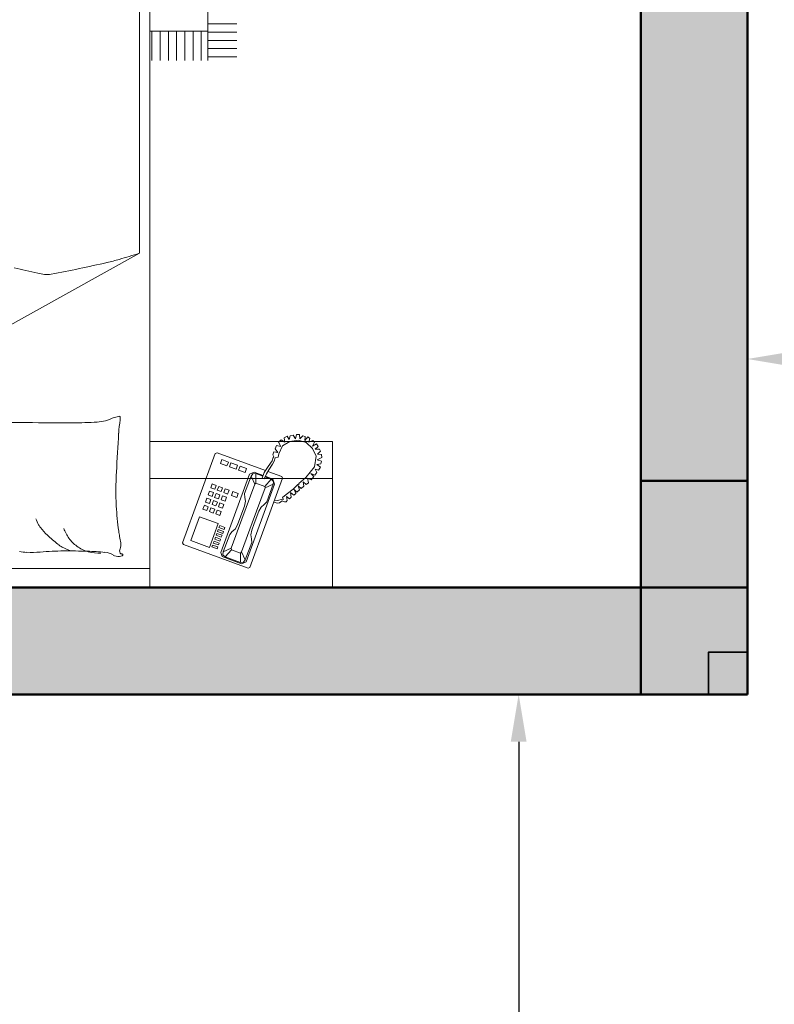
# Model space of a CAD drawing. Units: inches. Extents: x -7 to 1228, y -146 to 1091.
# Tile 37 of 88: x 1066 to 1129, y 34 to 117. Entities that reach past the tile are written whole.
import ezdxf

# ---------------------------------------------------------------- set-up
doc = ezdxf.new("R2010")
doc.units = ezdxf.units.IN
for name, color, linetype, lineweight in [('A-ANNO-DIMS', 2, 'Continuous', 18), ('A-COLS', 6, 'Continuous', 35), ('A-FURN', 8, 'Continuous', 18), ('A-WALL', 7, 'Continuous', 50), ('A-WALL-PATT', 251, 'Continuous', 13)]:
    doc.layers.add(name, color=color, linetype=linetype, lineweight=lineweight)
doc.styles.add('DIM_FONT', font='SIMPLEX.shx', dxfattribs={"width": 0.8})
doc.styles.get("Standard").update_dxf_attribs({"font": 'arial.ttf'})
doc.dimstyles.new('ISO-25', dxfattribs={"dimtxt": 7, "dimasz": 4, "dimexe": 1.25, "dimexo": 0.625, "dimtad": 1, "dimdec": 1, "dimlunit": 3, "dimtxsty": 'Standard', "dimcen": 2.5, "dimadec": 0, "dimazin": 0, "dimtfac": 1, "dimtdec": 1, "dimtmove": 1, "dimatfit": 3, "dimfxl": 1, "dimarcsym": 0})

# ---------------------------------------------------------------- blocks, each defined once
blk = doc.blocks.new('A$C4F634EDD')
for p, q in [((0.5, 2.6295), (2.3, 2.6295)), ((2.3, 2.6295), (2.3, 0.5295)), ((2.3, 2.6295), (2.8, 2.6295)), ((2.3, 2.2295), (2.3, 2.6295)), ((2.8, 2.6295), (2.8, 2.2295)), ((0.5, 2.5771), (2.3, 2.5771)), ((2.392, 2.5115), (2.5692, 2.5765)), ((2.4985, 2.5445), (2.5516, 2.564)), ((2.5516, 2.564), (2.5637, 2.5584)), ((2.5692, 2.5765), (2.574, 2.5743)), ((2.574, 2.5743), (2.6638, 2.3298)), ((2.4946, 2.5331), (2.4985, 2.5445)), ((2.5062, 2.5454), (2.5004, 2.5392)), ((2.5004, 2.5392), (2.5013, 2.5315)), ((2.5062, 2.5454), (2.5487, 2.561)), ((2.5235, 2.5256), (2.5062, 2.5454)), ((2.5483, 2.5347), (2.5487, 2.561)), ((2.5487, 2.561), (2.5571, 2.56)), ((2.5615, 2.5536), (2.5514, 2.5318)), ((2.5571, 2.56), (2.5615, 2.5536)), ((2.5615, 2.5536), (2.5791, 2.5058)), ((2.5637, 2.5584), (2.6418, 2.3458)), ((2.3898, 2.5066), (2.392, 2.5115)), ((2.412, 2.5007), (2.4634, 2.5196)), ((2.4634, 2.5196), (2.4875, 2.454)), ((2.4842, 2.5232), (2.47, 2.518)), ((2.47, 2.518), (2.472, 2.5127)), ((2.472, 2.5127), (2.4862, 2.5179)), ((2.4881, 2.5126), (2.4739, 2.5074)), ((2.4862, 2.5179), (2.4842, 2.5232)), ((2.4901, 2.5073), (2.4881, 2.5126)), ((2.5734, 2.3187), (2.4946, 2.5331)), ((2.5013, 2.5315), (2.5188, 2.4836)), ((2.5013, 2.5315), (2.5231, 2.5214)), ((2.5231, 2.5214), (2.5235, 2.5256)), ((2.5523, 2.4417), (2.5231, 2.5214)), ((2.5483, 2.5347), (2.5235, 2.5256)), ((2.5514, 2.5318), (2.5483, 2.5347)), ((2.5807, 2.4521), (2.5514, 2.5318)), ((2.4795, 2.2621), (2.3898, 2.5066)), ((2.4361, 2.4352), (2.412, 2.5007)), ((2.4739, 2.5074), (2.4759, 2.502)), ((2.4759, 2.502), (2.4901, 2.5073)), ((2.492, 2.5019), (2.4778, 2.4967)), ((2.4778, 2.4967), (2.4798, 2.4914)), ((2.4798, 2.4914), (2.494, 2.4966)), ((2.4959, 2.4913), (2.4817, 2.4861)), ((2.4817, 2.4861), (2.4837, 2.4808)), ((2.4837, 2.4808), (2.4979, 2.486)), ((2.494, 2.4966), (2.492, 2.5019)), ((2.4979, 2.486), (2.4959, 2.4913)), ((2.5188, 2.4836), (2.5256, 2.4761)), ((2.5788, 2.4956), (2.5767, 2.4848)), ((2.5767, 2.4848), (2.5795, 2.4717)), ((2.5791, 2.5058), (2.5788, 2.4956)), ((2.4998, 2.4807), (2.4856, 2.4755)), ((2.4856, 2.4755), (2.4876, 2.4702)), ((2.4876, 2.4702), (2.5018, 2.4754)), ((2.5037, 2.47), (2.4895, 2.4648)), ((2.4895, 2.4648), (2.4915, 2.4595)), ((2.4915, 2.4595), (2.5057, 2.4647)), ((2.5018, 2.4754), (2.4998, 2.4807)), ((2.5057, 2.4647), (2.5037, 2.47)), ((2.5256, 2.4761), (2.5342, 2.4692)), ((2.5342, 2.4692), (2.5405, 2.4574)), ((2.5405, 2.4574), (2.547, 2.4397)), ((2.5795, 2.4717), (2.586, 2.454)), ((2.4875, 2.454), (2.4361, 2.4352)), ((2.4811, 2.4276), (2.4917, 2.4315)), ((2.485, 2.4169), (2.4811, 2.4276)), ((2.4917, 2.4315), (2.4956, 2.4208)), ((2.5594, 2.4061), (2.547, 2.4397)), ((2.5523, 2.4417), (2.5875, 2.346)), ((2.5807, 2.4521), (2.6158, 2.3564)), ((2.5984, 2.4204), (2.586, 2.454)), ((2.4457, 2.4146), (2.4563, 2.4185)), ((2.4496, 2.4039), (2.4457, 2.4146)), ((2.4602, 2.4078), (2.4496, 2.4039)), ((2.4563, 2.4185), (2.4602, 2.4078)), ((2.4634, 2.4211), (2.474, 2.425)), ((2.4673, 2.4104), (2.4634, 2.4211)), ((2.4779, 2.4143), (2.4673, 2.4104)), ((2.4706, 2.4016), (2.4812, 2.4055)), ((2.4745, 2.3909), (2.4706, 2.4016)), ((2.474, 2.425), (2.4779, 2.4143)), ((2.4812, 2.4055), (2.4851, 2.3949)), ((2.4956, 2.4208), (2.485, 2.4169)), ((2.4883, 2.4081), (2.4989, 2.412)), ((2.4922, 2.3975), (2.4883, 2.4081)), ((2.5028, 2.4014), (2.4922, 2.3975)), ((2.4989, 2.412), (2.5028, 2.4014)), ((2.5622, 2.393), (2.5594, 2.4061)), ((2.6047, 2.4086), (2.5984, 2.4204)), ((2.6133, 2.4017), (2.6047, 2.4086)), ((2.6201, 2.3941), (2.6133, 2.4017)), ((2.4528, 2.3951), (2.4635, 2.399)), ((2.4567, 2.3844), (2.4528, 2.3951)), ((2.4674, 2.3883), (2.4567, 2.3844)), ((2.46, 2.3756), (2.4706, 2.3795)), ((2.4639, 2.365), (2.46, 2.3756)), ((2.4635, 2.399), (2.4674, 2.3883)), ((2.4706, 2.3795), (2.4745, 2.3689)), ((2.4851, 2.3949), (2.4745, 2.3909)), ((2.4777, 2.3821), (2.4883, 2.386)), ((2.4816, 2.3715), (2.4777, 2.3821)), ((2.4922, 2.3754), (2.4816, 2.3715)), ((2.4883, 2.386), (2.4922, 2.3754)), ((2.4954, 2.3886), (2.5061, 2.3925)), ((2.4993, 2.378), (2.4954, 2.3886)), ((2.51, 2.3819), (2.4993, 2.378)), ((2.5061, 2.3925), (2.51, 2.3819)), ((2.5238, 2.3769), (2.538, 2.3821)), ((2.5277, 2.3663), (2.5238, 2.3769)), ((2.538, 2.3821), (2.5419, 2.3715)), ((2.5598, 2.372), (2.5601, 2.3822)), ((2.5601, 2.3822), (2.5622, 2.393)), ((2.6376, 2.3463), (2.6201, 2.3941)), ((2.6499, 2.3979), (2.6397, 2.3953)), ((2.6417, 2.39), (2.6488, 2.391)), ((2.6488, 2.391), (2.6538, 2.3895)), ((2.6551, 2.397), (2.6499, 2.3979)), ((2.6538, 2.3895), (2.6596, 2.388)), ((2.6627, 2.392), (2.6551, 2.397)), ((2.6596, 2.388), (2.6626, 2.3867)), ((2.6626, 2.3867), (2.6662, 2.388)), ((2.6692, 2.394), (2.6627, 2.392)), ((2.6662, 2.388), (2.6632, 2.3828)), ((2.6632, 2.3828), (2.6736, 2.3744)), ((2.6736, 2.3944), (2.6692, 2.394)), ((2.6765, 2.391), (2.6736, 2.3944)), ((2.6736, 2.3744), (2.6922, 2.3593)), ((2.6742, 2.3795), (2.6765, 2.391)), ((2.6824, 2.3858), (2.6742, 2.3795)), ((2.6873, 2.3815), (2.6824, 2.3858)), ((2.6853, 2.369), (2.6873, 2.3815)), ((2.6946, 2.376), (2.6853, 2.369)), ((2.6995, 2.3713), (2.6946, 2.376)), ((2.4745, 2.3689), (2.4639, 2.365)), ((2.4672, 2.3561), (2.4778, 2.36)), ((2.4711, 2.3455), (2.4672, 2.3561)), ((2.4817, 2.3494), (2.4711, 2.3455)), ((2.4778, 2.36), (2.4817, 2.3494)), ((2.4849, 2.3626), (2.4955, 2.3665)), ((2.4888, 2.352), (2.4849, 2.3626)), ((2.4994, 2.3559), (2.4888, 2.352)), ((2.4955, 2.3665), (2.4994, 2.3559)), ((2.5026, 2.3691), (2.5132, 2.373)), ((2.5065, 2.3585), (2.5026, 2.3691)), ((2.5171, 2.3624), (2.5065, 2.3585)), ((2.5132, 2.373), (2.5171, 2.3624)), ((2.5419, 2.3715), (2.5277, 2.3663)), ((2.5774, 2.3242), (2.5598, 2.372)), ((2.6154, 2.3522), (2.5905, 2.3431)), ((2.6158, 2.3564), (2.6154, 2.3522)), ((2.6154, 2.3522), (2.6327, 2.3324)), ((2.6376, 2.3463), (2.6158, 2.3564)), ((2.6922, 2.3593), (2.7051, 2.3473)), ((2.695, 2.3603), (2.6995, 2.3713)), ((2.7031, 2.3682), (2.695, 2.3603)), ((2.7096, 2.3616), (2.7031, 2.3682)), ((2.7051, 2.3473), (2.7079, 2.3475)), ((2.7062, 2.351), (2.7096, 2.3616)), ((2.7147, 2.3578), (2.7062, 2.351)), ((2.7079, 2.3475), (2.7079, 2.3443)), ((2.7214, 2.3517), (2.7147, 2.3578)), ((2.7196, 2.34), (2.7214, 2.3517)), ((2.7286, 2.3466), (2.7196, 2.34)), ((2.7346, 2.3423), (2.7286, 2.3466)), ((2.8, 2.3301), (2.3, 2.3301)), ((2.5774, 2.3242), (2.5875, 2.346)), ((2.5818, 2.3178), (2.5774, 2.3242)), ((2.6104, 2.3222), (2.5855, 2.3131)), ((2.5875, 2.346), (2.5905, 2.3431)), ((2.5905, 2.3431), (2.5901, 2.3168)), ((2.5901, 2.3168), (2.6097, 2.324)), ((2.613, 2.3312), (2.6077, 2.3293)), ((2.6077, 2.3293), (2.6135, 2.3141)), ((2.6192, 2.3174), (2.613, 2.3312)), ((2.6153, 2.3261), (2.6327, 2.3324)), ((2.6369, 2.332), (2.6161, 2.3243)), ((2.6616, 2.3249), (2.6234, 2.3109)), ((2.6327, 2.3324), (2.6385, 2.3386)), ((2.6418, 2.3458), (2.6369, 2.332)), ((2.6385, 2.3386), (2.6376, 2.3463)), ((2.6638, 2.3298), (2.6616, 2.3249)), ((2.7079, 2.3443), (2.727, 2.3277)), ((2.727, 2.3277), (2.7512, 2.2983)), ((2.732, 2.3295), (2.7346, 2.3423)), ((2.7423, 2.3345), (2.732, 2.3295)), ((2.7406, 2.3172), (2.7495, 2.325)), ((2.7519, 2.3218), (2.7406, 2.3172)), ((2.7495, 2.325), (2.7423, 2.3345)), ((2.7575, 2.3144), (2.7519, 2.3218)), ((2.6172, 2.3086), (2.4844, 2.2599)), ((2.5114, 2.2959), (2.4936, 2.2894)), ((2.5153, 2.2853), (2.5114, 2.2959)), ((2.5362, 2.305), (2.5185, 2.2985)), ((2.5185, 2.2985), (2.5224, 2.2879)), ((2.5224, 2.2879), (2.5401, 2.2944)), ((2.5401, 2.2944), (2.5362, 2.305)), ((2.561, 2.3141), (2.5433, 2.3076)), ((2.5433, 2.3076), (2.5472, 2.297)), ((2.5472, 2.297), (2.5649, 2.3035)), ((2.5649, 2.3035), (2.561, 2.3141)), ((2.5855, 2.3131), (2.5734, 2.3187)), ((2.5901, 2.3168), (2.5818, 2.3178)), ((2.6135, 2.3141), (2.6244, 2.2977)), ((2.626, 2.3069), (2.6192, 2.3174)), ((2.6244, 2.2977), (2.6349, 2.2825)), ((2.6365, 2.2916), (2.626, 2.3069)), ((2.7512, 2.2983), (2.756, 2.2695)), ((2.7526, 2.3045), (2.7575, 2.3144)), ((2.7622, 2.308), (2.7526, 2.3045)), ((2.7574, 2.2924), (2.7673, 2.2997)), ((2.7673, 2.2997), (2.7622, 2.308)), ((2.4936, 2.2894), (2.4976, 2.2788)), ((2.4976, 2.2788), (2.5153, 2.2853)), ((2.6349, 2.2825), (2.638, 2.273)), ((2.6407, 2.2834), (2.6365, 2.2916)), ((2.6399, 2.2712), (2.6374, 2.2659)), ((2.6374, 2.2659), (2.6398, 2.257)), ((2.638, 2.273), (2.6399, 2.2712)), ((2.6438, 2.2739), (2.6407, 2.2834)), ((2.6519, 2.2716), (2.6438, 2.2739)), ((2.6535, 2.2628), (2.6519, 2.2716)), ((2.756, 2.2695), (2.7459, 2.2483)), ((2.7687, 2.2905), (2.7574, 2.2924)), ((2.7587, 2.279), (2.7699, 2.2828)), ((2.7708, 2.2725), (2.7587, 2.279)), ((2.7699, 2.2828), (2.7687, 2.2905)), ((2.7706, 2.2643), (2.7708, 2.2725)), ((2.4844, 2.2599), (2.4795, 2.2621)), ((2.6398, 2.257), (2.6509, 2.259)), ((2.6509, 2.259), (2.6431, 2.2492)), ((2.6431, 2.2492), (2.6473, 2.2398)), ((2.6473, 2.2398), (2.6592, 2.2429)), ((2.6592, 2.2429), (2.6521, 2.2314)), ((2.6636, 2.2409), (2.6535, 2.2628)), ((2.6836, 2.2287), (2.6636, 2.2409)), ((2.7459, 2.2483), (2.7284, 2.2317)), ((2.7509, 2.2314), (2.7459, 2.2418)), ((2.7459, 2.2418), (2.7568, 2.2352)), ((2.7529, 2.2505), (2.7645, 2.2498)), ((2.7607, 2.2424), (2.7529, 2.2505)), ((2.7568, 2.2352), (2.7607, 2.2424)), ((2.759, 2.2637), (2.7706, 2.2643)), ((2.7676, 2.2559), (2.759, 2.2637)), ((2.7645, 2.2498), (2.7676, 2.2559)), ((2.8, 2.2295), (2.3, 2.2295)), ((2.6521, 2.2314), (2.6598, 2.2248)), ((2.6598, 2.2248), (2.6697, 2.2309)), ((2.6697, 2.2309), (2.6684, 2.219)), ((2.6684, 2.219), (2.6761, 2.2145)), ((2.6761, 2.2145), (2.6821, 2.2237)), ((2.6821, 2.2237), (2.6843, 2.2135)), ((2.7063, 2.2256), (2.6836, 2.2287)), ((2.6843, 2.2135), (2.6927, 2.2117)), ((2.6927, 2.2117), (2.6986, 2.222)), ((2.6986, 2.222), (2.7019, 2.2098)), ((2.7284, 2.2317), (2.7063, 2.2256)), ((2.7102, 2.2104), (2.7113, 2.2218)), ((2.7113, 2.2218), (2.7192, 2.2137)), ((2.7192, 2.2137), (2.7255, 2.2152)), ((2.7255, 2.2152), (2.7242, 2.2265)), ((2.7242, 2.2265), (2.7324, 2.2165)), ((2.7324, 2.2165), (2.7386, 2.2208)), ((2.7386, 2.2208), (2.7354, 2.2306)), ((2.7354, 2.2306), (2.7462, 2.2264)), ((2.7462, 2.2264), (2.7509, 2.2314)), ((2.7019, 2.2098), (2.7102, 2.2104)), ((1.5035, 2.141), (2.2716, 1.7136)), ((2.2716, 0.5617), (2.2716, 1.7136)), ((2.3061, 1.1052), (2.3061, 1.1852)), ((2.3286, 1.1052), (2.3286, 1.1852)), ((2.3511, 1.1052), (2.3511, 1.1852)), ((2.3736, 1.1052), (2.3736, 1.1852)), ((2.3961, 1.1052), (2.3961, 1.1852)), ((2.4186, 1.1052), (2.4186, 1.1852)), ((2.4411, 1.1052), (2.4411, 1.1852)), ((2.4588, 1.1852), (2.4588, 0)), ((2.4588, 1.1753), (2.5388, 1.1753)), ((2.4588, 1.1528), (2.5388, 1.1528)), ((2.4588, 1.1303), (2.5388, 1.1303)), ((2.4588, 1.1078), (2.5388, 1.1078)), ((2.3, 1.1052), (2.4588, 1.1052)), ((2.4588, 1.0853), (2.5388, 1.0853))]:
    blk.add_line(p, q)
for centre, radius, start, end in [((2.1724, 2.5864), 0.0539, 275.2592, 300.6513), ((2.2146, 2.5152), 0.0289, 85.6975, 120.6513), ((2.2149, 2.519), 0.0251, 68.2117, 85.6975), ((2.2226, 2.533), 0.00428, 78.1069, 158.0096), ((2.224, 2.5395), 0.00232, 258.1069, 19.564), ((2.2229, 2.5391), 0.00342, 19.564, 68.2117), ((1.97, 2.3805), 0.1524, 92.5386, 100.1899), ((1.9761, 2.2433), 0.2897, 85.1982, 92.5386), ((2.0734, 3.4021), 0.8732, 265.1982, 269.4243), ((2.291, 2.2032), 0.3916, 128.3886, 133.8115), ((2.0954, 2.45), 0.0768, 117.2396, 128.3886), ((2.1674, 2.3102), 0.234, 110.8603, 117.2396), ((2.0797, 4.0232), 1.4943, 269.4243, 271.9079), ((2.1588, 2.4357), 0.0992, 126.0864, 143.8234), ((2.1588, 2.4357), 0.0992, 105.9352, 126.0864), ((2.1021, 3.3501), 0.8208, 271.9079, 275.2592), ((2.1588, 2.4357), 0.0992, 85.7841, 105.9352), ((2.2331, 2.5288), 0.0156, 158.0096, 201.421), ((2.1881, 2.5111), 0.0328, 351.8665, 21.421), ((2.1757, 2.3233), 0.2252, 133.8115, 140.9651), ((2.1588, 2.4357), 0.0992, 143.8234, 161.5603), ((2.4114, 2.448), 0.1983, 167.8905, 172.3191), ((1.977, 2.5413), 0.246, 347.8905, 351.8665), ((2.1719, 2.3625), 0.2002, 151.6832, 156.9972), ((2.0391, 2.4341), 0.0493, 140.9651, 151.6832), ((3.1198, 2.3525), 0.9131, 172.3191, 176.6313), ((2.8858, 2.3663), 0.6787, 176.6313, 181.6331), ((3.5721, 2.3859), 1.3652, 181.6331, 183.055), ((15.8249, 3.0398), 13.6356, 183.05496, 183.50486), ((2.5355, 2.2258), 0.3212, 183.5049, 189.9984), ((2.1093, -19.8405), 22.0183, 90.37908, 91.01965), ((2.0605, -3.5404), 5.7185, 89.7135, 90.9704), ((2.0833, 1.0141), 1.164, 86.426, 89.7135), ((2.1467, 2.0302), 0.1459, 77.131, 86.426), ((2.1691, 2.1283), 0.0453, 62.7159, 77.131), ((2.2251, 2.2367), 0.0767, 242.7159, 253.7788), ((2.2281, 2.247), 0.0875, 253.7788, 262.8796), ((2.2174, 2.1615), 0.00132, 262.8796, 343.3022), ((2.2001, 2.1667), 0.0193, 343.3022, 9.9984), ((1.4194, 4.2174), 2.5158, 281.6741, 283.1904), ((2.0378, 1.5789), 0.1942, 97.7304, 103.1904), ((2.0195, 1.7137), 0.0581, 79.2724, 97.7304), ((1.2737, -2.2227), 4.0646, 77.0745, 79.2724), ((2.0359, 1.0981), 0.6574, 74.0648, 77.0745), ((1.7125, -0.0344), 1.8351, 72.2636, 74.0648)]:
    blk.add_arc(centre, radius, start, end)
at = {"style": 'DIM_FONT', "width": 0.8, "flags": 9}
for tag, p in [('YSIZE', (0.5, 2.6295)), ('XSIZE', (0.5, 2.6295)), ('XSIZE', (2.2985, 2.6295)), ('YSIZE', (2.2985, 2.6295))]:
    blk.add_attdef(tag, p, '', height=0.0005, dxfattribs=at)
blk = doc.blocks.new('*D16')
at = {"layer": 'A-ANNO-DIMS', "color": 0, "lineweight": -2, "transparency": 16777216}
for p, q in [((1127, 88.082), (1127, 87.038)), ((1131, 88.288), (1183, 88.288)), ((1187, 88.082), (1187, 87.038))]:
    blk.add_line(p, q, dxfattribs=at)
at = {"layer": 'A-ANNO-DIMS', "color": 0, "transparency": 16777216}
for points in [[(1131, 88.955), (1131, 87.622), (1127, 88.288)], [(1183, 88.955), (1183, 87.622), (1187, 88.288)]]:
    blk.add_solid(points, dxfattribs=at)
at = {"layer": 'Defpoints', "color": 0, "transparency": 16777216}
for p in [(1127, 88.707), (1187, 88.707), (1187, 88.288)]:
    blk.add_point(p, dxfattribs=at)
at = {"layer": 'A-ANNO-DIMS', "color": 0, "transparency": 16777216, "insert": (1157, 92.473), "char_height": 7, "attachment_point": 5}
blk.add_mtext("5'", dxfattribs=at)
blk = doc.blocks.new('*D17')
at = {"layer": 'A-ANNO-DIMS', "color": 0, "lineweight": -2, "transparency": 16777216}
for p, q in [((1108.337, 60), (1108.962, 60)), ((1107.712, 56), (1107.712, 4)), ((1108.337, 0), (1108.962, 0))]:
    blk.add_line(p, q, dxfattribs=at)
at = {"layer": 'A-ANNO-DIMS', "color": 0, "transparency": 16777216}
for points in [[(1107.046, 56), (1108.379, 56), (1107.712, 60)], [(1107.046, 4), (1108.379, 4), (1107.712, 0)]]:
    blk.add_solid(points, dxfattribs=at)
at = {"layer": 'Defpoints', "color": 0, "transparency": 16777216}
for p in [(1107.712, 60), (1107.712, 0), (1107.712, 0)]:
    blk.add_point(p, dxfattribs=at)
at = {"layer": 'A-ANNO-DIMS', "color": 0, "transparency": 16777216, "insert": (1103.528, 30), "char_height": 7, "attachment_point": 5, "rotation": 90}
blk.add_mtext("5'", dxfattribs=at)

msp = doc.modelspace()

# ---------------------------------------------------------------- hatches: boundary and pattern name
at = {"layer": 'A-COLS'}
h = msp.add_hatch(color=256, dxfattribs=at)
h.dxf.hatch_style = 1
h.paths.add_polyline_path([(1127, 78), (1118, 78), (1118, 60), (1123.711, 60), (1123.711, 63.546), (1127, 63.546)])
h = msp.add_hatch(color=256, dxfattribs=at)
h.dxf.hatch_style = 1
h.paths.add_polyline_path([(1123.711, 63.546), (1123.711, 60), (1127, 60), (1127, 63.546)])
at = {"layer": 'A-WALL-PATT'}
h = msp.add_hatch(color=256, dxfattribs=at)
h.dxf.hatch_style = 1
h.paths.add_polyline_path([(69, 568), (60, 568), (60, 493), (63.289, 493), (69, 493)])
h.paths.add_polyline_path([(69, 662.405), (60, 662.405), (60, 586), (69, 586)], flags=17)
h.paths.add_polyline_path([(69, 723), (184, 723), (184, 734), (179, 734), (179, 728), (69, 728), (69, 741.623), (60, 741.623), (60, 698.405), (69, 698.405)], flags=17)
h.paths.add_polyline_path([(69, 782), (231, 782), (231, 728), (231, 723), (231, 586), (236, 586), (236, 787), (69, 787), (69, 800.126), (60, 800.126), (60, 765.623), (69, 765.623)])
h.paths.add_polyline_path([(184, 842), (189, 842), (189, 848), (173, 848), (173, 842), (179, 842), (179, 787), (184, 787)])
h.paths.add_polyline_path([(118.22, 69), (69, 69), (69, 60), (118.22, 60)])
h.paths.add_polyline_path([(227, 69), (154.22, 69), (154.22, 60), (227, 60)])
h.paths.add_polyline_path([(236, 60), (232.711, 60), (227, 60), (227, 36), (236, 36)])
h.paths.add_polyline_path([(389, 60), (380, 60), (380, 36), (389, 36)])
h.paths.add_polyline_path([(384, 181), (380, 181), (380, 115), (380, 78), (384, 78)])
h.paths.add_polyline_path([(380, 115), (334.547, 115), (334.547, 109), (380, 109)])
h.paths.add_polyline_path([(274.547, 115), (236, 115), (236, 201), (232.711, 201), (231, 201), (231, 78), (236, 78), (236, 109), (274.547, 109)])
h.paths.add_polyline_path([(69, 123), (60, 123), (60, 78), (69, 78)])
h.paths.add_polyline_path([(69, 201), (60, 201), (60, 159), (69, 159)])
h.paths.add_polyline_path([(143, 219), (69, 219), (69, 213), (143, 213)], flags=17)
h.paths.add_polyline_path([(189, 219), (184, 219), (184, 274), (231, 274), (231, 219), (236, 219), (236, 279), (184, 279), (184, 297), (179, 297), (179, 279), (69, 279), (69, 290.912), (60, 290.912), (60, 262.179), (69, 262.179), (69, 274), (179, 274), (179, 219), (173, 219), (173, 213), (189, 213)])
h.paths.add_polyline_path([(69, 238.179), (60, 238.179), (60, 219), (69, 219)], flags=17)
h.paths.add_polyline_path([(69, 333), (60, 333), (60, 314.912), (69, 314.912), (69, 316.965)])
h.paths.add_polyline_path([(190, 338), (184, 338), (69, 338), (69, 333), (179, 333), (179, 327), (184, 327), (184, 333.021), (190, 333.046)])
h.paths.add_polyline_path([(69, 386.806), (60, 386.806), (60, 351), (69, 351)])
h.paths.add_polyline_path([(69, 475), (60, 475), (60, 422.806), (69, 422.806)])
h.paths.add_polyline_path([(236, 475), (231, 475), (231, 351.238), (236, 351.238)])
h.paths.add_polyline_path([(384, 475), (380, 475), (380, 362), (384, 362)])
h.paths.add_polyline_path([(547, 307), (439, 307), (439, 356), (445, 356), (445, 362), (433, 362), (433, 307), (380, 307), (380, 244), (380, 241), (384, 241), (384, 301), (433, 301), (433, 277), (439, 277), (439, 301), (547, 301)])
h.paths.add_polyline_path([(547, 241), (439, 241), (439, 247), (433, 247), (433, 235), (547, 235)])
h.paths.add_polyline_path([(450, 69), (440.286, 69), (424.889, 69), (389, 69), (389, 60), (450, 60)])
h.paths.add_polyline_path([(547, 69), (486, 69), (486, 60), (547, 60)])
h.paths.add_polyline_path([(556, 148.268), (547, 148.268), (547, 78), (556, 78)])
h.paths.add_polyline_path([(556, 223), (547, 223), (547, 195), (547, 184.268), (556, 184.268)])
h.paths.add_polyline_path([(556, 311.192), (547, 311.192), (547, 273.075), (556, 273.075)])
h.paths.add_polyline_path([(556, 344), (552.711, 344), (547, 344), (547, 335.192), (556, 335.192)])
h.paths.add_polyline_path([(556, 249.075), (547, 249.075), (547, 241), (556, 241)])
h.paths.add_polyline_path([(547, 362), (475, 362), (475, 356), (547, 356)], flags=0)
h.paths.add_polyline_path([(556, 399.621), (547, 399.621), (547, 362), (556, 362)])
h.paths.add_polyline_path([(556, 475), (547, 475), (547, 435.621), (556, 435.621)])
h.paths.add_polyline_path([(547, 493), (389, 493), (389, 487), (547, 487)])
h.paths.add_polyline_path([(380, 493), (278, 493), (278, 487), (380, 487)])
h.paths.add_polyline_path([(227, 493), (69, 493), (69, 487), (227, 487)])
h.paths.add_polyline_path([(643, 122.445), (634, 122.445), (634, 78), (643, 78)])
h.paths.add_polyline_path([(702.5, 69), (692.786, 69), (677.389, 69), (643, 69), (643, 60), (702.5, 60)])
h.paths.add_polyline_path([(798, 69), (738.5, 69), (738.5, 60), (798, 60)])
h.paths.add_polyline_path([(807, 60), (803.711, 60), (798, 60), (798, 36), (807, 36)])
h.paths.add_polyline_path([(807, 109), (846.751, 109), (846.751, 115), (807, 115), (807, 159), (802, 159), (802, 78), (807, 78)])
h.paths.add_polyline_path([(807, 201), (802, 201), (802, 195), (807, 195)])
h.paths.add_polyline_path([(643, 201), (634, 201), (634, 158.445), (643, 158.445)])
h.paths.add_polyline_path([(756, 225), (751, 225), (751, 219), (643, 219), (643, 213), (756, 213)])
h.paths.add_polyline_path([(643, 240.848), (634, 240.848), (634, 219), (643, 219)])
h.paths.add_polyline_path([(643, 274), (643, 288.629), (634, 288.629), (634, 264.848), (643, 264.848)])
h.paths.add_polyline_path([(802, 279), (756, 279), (756, 297), (751, 297), (751, 279), (643, 279), (643, 274), (751, 274), (751, 255), (756, 255), (756, 274), (802, 274)])
h.paths.add_polyline_path([(807, 333), (803.711, 333), (802, 333), (802, 279), (802, 274), (802, 219), (807, 219)])
h.paths.add_polyline_path([(956, 182), (951, 182), (951, 115), (906.751, 115), (906.751, 109), (951, 109), (951, 78), (956, 78)])
h.paths.add_polyline_path([(960, 60), (951, 60), (951, 36), (960, 36)])
h.paths.add_polyline_path([(1021, 69), (1005.781, 69), (960, 69), (960, 60), (1021, 60)])
h.paths.add_polyline_path([(956, 224), (951, 224), (951, 218), (956, 218)])
h.paths.add_polyline_path([(956, 302), (1004, 302), (1004, 278), (1010, 278), (1010, 302), (1118, 302), (1118, 290.809), (1127, 290.809), (1127, 326.968), (1118, 326.968), (1118, 320.966), (1118, 307), (1010, 307), (1010, 356), (1016, 356), (1016, 362), (1004, 362), (1004, 307), (951, 307), (951, 244), (951, 242), (954.289, 242), (956, 242)])
h.paths.add_polyline_path([(643, 333), (634, 333), (634, 312.629), (643, 312.629), (643, 316.965)])
h.paths.add_polyline_path([(756, 338), (643, 338), (643, 333), (751, 333), (751, 327), (756, 327)])
h.paths.add_polyline_path([(643, 388), (634, 388), (634, 351), (643, 351)])
h.paths.add_polyline_path([(807, 357), (802, 357), (802, 351), (807, 351)])
h.paths.add_polyline_path([(807, 475), (802, 475), (802, 393), (807, 393)])
h.paths.add_polyline_path([(643, 475), (634, 475), (634, 424), (643, 424)])
h.paths.add_polyline_path([(798, 493), (643, 493), (643, 487), (798, 487)])
h.paths.add_polyline_path([(634, 493), (556, 493), (556, 487), (634, 487)])
h.paths.add_polyline_path([(813, 493), (807, 493), (807, 487), (813, 487)])
h.paths.add_polyline_path([(951, 493), (849, 493), (849, 487), (951, 487)])
h.paths.add_polyline_path([(956, 484), (951, 484), (951, 374), (956, 374)])
h.paths.add_polyline_path([(1109, 493), (969, 493), (969, 487), (1109, 487)])
h.paths.add_polyline_path([(1127, 484), (1118, 484), (1118, 450.641), (1127, 450.641)])
h.paths.add_polyline_path([(1127, 414.641), (1118, 414.641), (1118, 365), (1127, 365)])
h.paths.add_polyline_path([(1109, 362), (1046, 362), (1046, 356), (1109, 356)], flags=17)
h.paths.add_polyline_path([(1127, 356), (1123.454, 356), (1118, 356), (1118, 350.968), (1127, 350.968)], flags=0)
h.paths.add_polyline_path([(1127, 266.809), (1118, 266.809), (1118, 262.361), (1118, 242), (1127, 242)], flags=17)
h.paths.add_polyline_path([(1118, 242), (1010, 242), (1010, 248), (1004, 248), (1004, 237), (1118, 237)])
h.paths.add_polyline_path([(1127, 224), (1118, 224), (1118, 170), (1127, 170)])
h.paths.add_polyline_path([(1127, 134), (1118, 134), (1118, 78), (1127, 78)])
h.paths.add_polyline_path([(1118, 69), (1057, 69), (1057, 60), (1118, 60)])
h.paths.add_polyline_path([(227, 571.546), (227, 574), (69, 574), (69, 568), (227, 568)])
h.paths.add_polyline_path([(380, 571.546), (380, 574), (278, 574), (278, 568), (380, 568)])
h.paths.add_polyline_path([(242, 574), (236, 574), (236, 568), (242, 568)])
h.paths.add_polyline_path([(547, 571.546), (547, 574), (389, 574), (389, 568), (547, 568)])
h.paths.add_polyline_path([(384, 733), (380, 733), (380, 586), (384, 586)])
h.paths.add_polyline_path([(556, 646), (634, 646), (634, 655), (547, 655), (547, 586), (556, 586)])
h.paths.add_polyline_path([(634, 574), (556, 574), (556, 568), (634, 568)])
h.paths.add_polyline_path([(643, 655), (634, 655), (634, 586), (643, 586)])
h.paths.add_polyline_path([(798, 574), (643, 574), (643, 568), (798, 568)])
h.paths.add_polyline_path([(643, 663.854), (634, 663.854), (634, 655), (643, 655)])
h.paths.add_polyline_path([(556, 676.967), (547, 676.967), (547, 655), (556, 655)])
h.paths.add_polyline_path([(556, 733), (547, 733), (547, 712.967), (556, 712.967)])
h.paths.add_polyline_path([(643, 710), (634, 710), (634, 699.854), (643, 699.854)])
h.paths.add_polyline_path([(807, 668), (802, 668), (802, 586), (807, 586)])
h.paths.add_polyline_path([(951, 574), (849, 574), (849, 568), (951, 568)])
h.paths.add_polyline_path([(956, 691), (951, 691), (951, 577), (956, 577)])
h.paths.add_polyline_path([(1109, 574), (969, 574), (969, 568), (1109, 568)])
h.paths.add_polyline_path([(1127, 643.403), (1118, 643.403), (1118, 577), (1127, 577)])
h.paths.add_polyline_path([(1127, 568), (1123.454, 568), (1118, 568), (1118, 493), (1127, 493)])
h.paths.add_polyline_path([(1127, 733), (1118, 733), (1118, 679.403), (1127, 679.403)])
h.paths.add_polyline_path([(1127, 777.348), (1118, 777.348), (1118, 770.035), (1118, 751), (1127, 751)], flags=17)
h.paths.add_polyline_path([(1118, 751), (1010, 751), (1010, 757), (1004, 757), (1004, 745), (1118, 745)])
h.paths.add_polyline_path([(956, 811), (1004, 811), (1004, 787), (1010, 787), (1010, 811), (1017.874, 811), (1017.874, 811.627, -0.414214), (1018.247, 812), (1031.978, 812, -0.414214), (1032.351, 811.627), (1032.351, 811), (1118, 811), (1118, 801.348), (1127, 801.348), (1127, 834.685), (1118, 834.685), (1118, 830.238), (1118, 817), (1010, 817), (1010, 866), (1016, 866), (1016, 872), (1004, 872), (1004, 817), (956, 817), (956, 866), (951, 866), (951, 751), (954.289, 751), (956, 751)])
h.paths.add_polyline_path([(1118, 872), (1046, 872), (1046, 866), (1118, 866)], flags=17)
h.paths.add_polyline_path([(1127, 924.711), (1118, 924.711), (1118, 884), (1127, 884)])
h.paths.add_polyline_path([(1127, 866), (1123.711, 866), (1118, 866), (1118, 858.685), (1127, 858.685)], flags=17)
h.paths.add_polyline_path([(956, 983), (951, 983), (951, 952), (807, 952), (807, 983), (802, 983), (802, 902), (807, 902), (807, 946), (951, 946), (951, 884), (956, 884)])
h.paths.add_polyline_path([(807, 842), (802, 842), (802, 787), (756, 787), (756, 806), (751, 806), (751, 787), (643, 787), (643, 782), (751, 782), (751, 764), (756, 764), (756, 782), (802, 782), (802, 728), (807, 728)])
h.paths.add_polyline_path([(756, 848), (643, 848), (643, 842), (751, 842), (751, 836), (756, 836)])
h.paths.add_polyline_path([(756, 734), (751, 734), (751, 728), (643, 728), (643, 723), (756, 723)])
h.paths.add_polyline_path([(643, 749.791), (634, 749.791), (634, 728), (637.289, 728), (643, 728)])
h.paths.add_polyline_path([(643, 805.405), (634, 805.405), (634, 773.791), (643, 773.791)])
h.paths.add_polyline_path([(643, 896.663), (634, 896.663), (634, 860), (637.289, 860), (643, 860)])
h.paths.add_polyline_path([(643, 842), (634, 842), (634, 829.405), (643, 829.405)])
h.paths.add_polyline_path([(643, 983), (634, 983), (634, 932.663), (643, 932.663)])
h.paths.add_polyline_path([(1127, 983), (1118, 983), (1118, 960.711), (1127, 960.711)])
h.paths.add_polyline_path([(1118, 1001), (1077.525, 1001), (1077.525, 992), (1118, 992)])
h.paths.add_polyline_path([(1041.525, 1001), (960, 1001), (960, 992), (1041.525, 992)])
h.paths.add_polyline_path([(960, 1025), (951, 1025), (951, 1001), (954.289, 1001), (960, 1001)])
h.paths.add_polyline_path([(807, 1025), (798, 1025), (798, 1001), (807, 1001)])
h.paths.add_polyline_path([(798, 1001), (738.5, 1001), (738.5, 992), (798, 992)])
h.paths.add_polyline_path([(702.5, 1001), (643, 1001), (643, 992), (702.5, 992)])
h.paths.add_polyline_path([(547, 1001), (499.113, 1001), (499.113, 992), (547, 992)])
h.paths.add_polyline_path([(463.113, 1001), (389, 1001), (389, 992), (463.113, 992)])
h.paths.add_polyline_path([(389, 1025), (380, 1025), (380, 1022), (380, 1001), (383.289, 1001), (389, 1001)])
h.paths.add_polyline_path([(236, 1025), (227, 1025), (227, 1001), (236, 1001)])
h.paths.add_polyline_path([(236, 983), (231, 983), (231, 860), (236, 860)])
h.paths.add_polyline_path([(274.547, 952), (236, 952), (236, 946), (274.547, 946)])
h.paths.add_polyline_path([(380, 952), (334.547, 952), (334.547, 946), (380, 946)])
h.paths.add_polyline_path([(384, 983), (380, 983), (380, 884), (383.289, 884), (384, 884)])
h.paths.add_polyline_path([(227, 1001), (155.012, 1001), (155.012, 992), (162.875, 992), (227, 992)])
h.paths.add_polyline_path([(119.012, 1001), (69, 1001), (69, 992), (119.012, 992)])
h.paths.add_polyline_path([(69, 983), (60, 983), (60, 922.987), (69, 922.987)])
h.paths.add_polyline_path([(69, 886.987), (60, 886.987), (60, 860), (63.289, 860), (69, 860)])
h.paths.add_polyline_path([(143, 848), (69, 848), (69, 842), (143, 842)])

# ---------------------------------------------------------------- linework, layer by layer
at = {"layer": 'A-COLS'}
msp.add_lwpolyline([(1127, 60), (1123.711, 60), (1123.711, 63.546), (1127, 63.546)], close=True, dxfattribs=at)
at = {"layer": 'A-WALL'}
for p, q in [((1127, 60), (1127, 1001)), ((1118, 60), (1118, 302)), ((1118, 244), (1118, 60)), ((1118, 60), (1118, 78)), ((1118, 78), (1127, 78)), ((1127, 78), (1127, 60)), ((1127, 69), (951, 69)), ((1127, 60), (951, 60)), ((951, 60), (1127, 60)), ((1127, 60), (1118, 60))]:
    msp.add_line(p, q, dxfattribs=at)

# ---------------------------------------------------------------- block references
at = {"layer": 'A-FURN', "xscale": -30.79356024027943, "yscale": 30.79356024027943, "zscale": 30.79356024027943, "rotation": 180}
msp.add_blockref('A$C4F634EDD', (1005.781, 149.972), dxfattribs=at)

# ---------------------------------------------------------------- dimensions: what is measured, and where the dimension line sits
at = {"layer": 'A-ANNO-DIMS'}
dim = msp.add_linear_dim(base=(1187, 88.288), p1=(1127, 88.707), p2=(1187, 88.707), dimstyle='ISO-25', override={"dimclrd": 0, "dimclre": 0, "dimclrt": 0}, dxfattribs=at)
dim.commit()
dim.dimension.update_dxf_attribs({"geometry": '*D16', "text_midpoint": (1157, 92.473)})
dim = msp.add_linear_dim(base=(1107.712, 0), p1=(1107.712, 60), p2=(1107.712, 0), angle=90, dimstyle='ISO-25', override={"dimclrd": 0, "dimclre": 0, "dimclrt": 0}, dxfattribs=at)
dim.commit()
dim.dimension.update_dxf_attribs({"geometry": '*D17', "text_midpoint": (1103.528, 30)})

doc.saveas('drawing.dxf')
